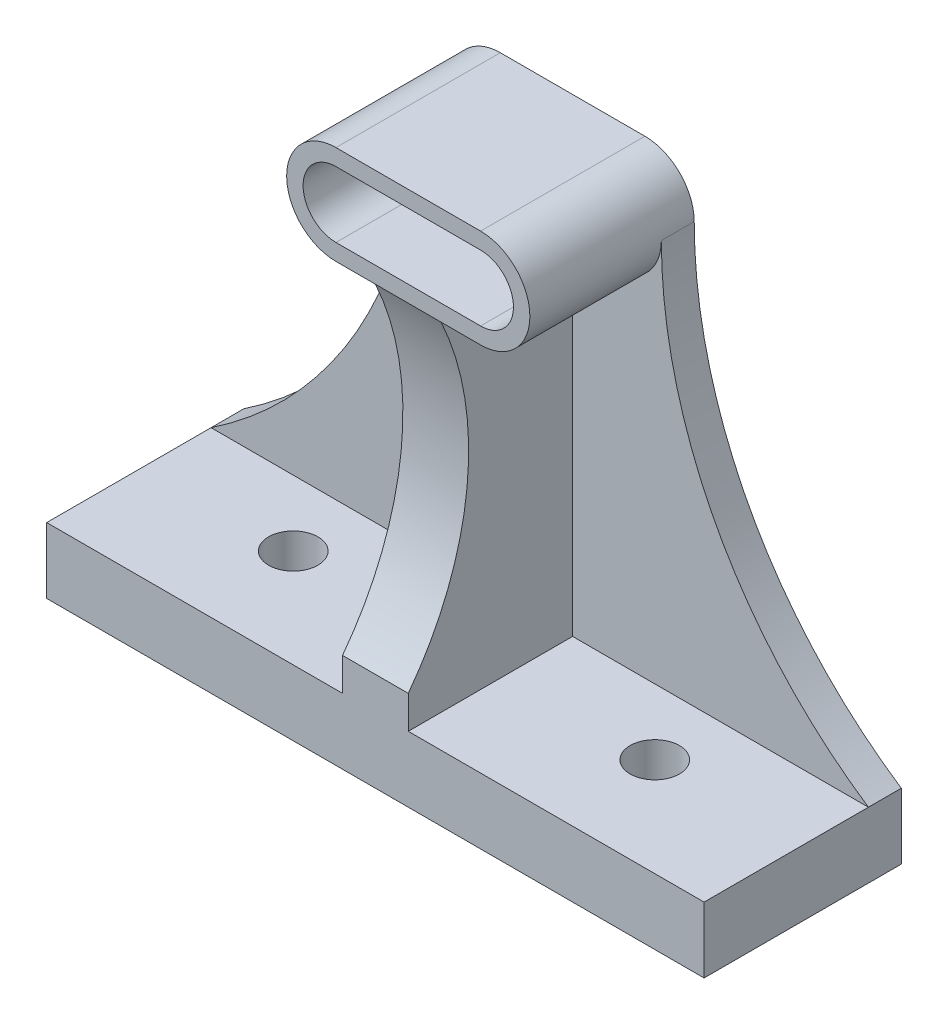
ISO-10303-21;
HEADER;
FILE_DESCRIPTION(('STEP AP214'),'2;1');
FILE_NAME('part.step','',(''),(''),'','','');
FILE_SCHEMA(('AUTOMOTIVE_DESIGN { 1 0 10303 214 1 1 1 1 }'));
ENDSEC;
DATA;
#1=APPLICATION_CONTEXT('core data for automotive mechanical design processes');
#2=APPLICATION_PROTOCOL_DEFINITION('international standard','automotive_design',2000,#1);
#3=PRODUCT_CONTEXT('',#1,'mechanical');
#4=PRODUCT('Part','Part','',(#3));
#5=PRODUCT_RELATED_PRODUCT_CATEGORY('part','',(#4));
#6=PRODUCT_DEFINITION_FORMATION('','',#4);
#7=PRODUCT_DEFINITION_CONTEXT('part definition',#1,'design');
#8=PRODUCT_DEFINITION('design','',#6,#7);
#9=PRODUCT_DEFINITION_SHAPE('','',#8);
#10=(LENGTH_UNIT() NAMED_UNIT(*) SI_UNIT(.MILLI.,.METRE.));
#11=(NAMED_UNIT(*) PLANE_ANGLE_UNIT() SI_UNIT($,.RADIAN.));
#12=(NAMED_UNIT(*) SI_UNIT($,.STERADIAN.) SOLID_ANGLE_UNIT());
#13=UNCERTAINTY_MEASURE_WITH_UNIT(LENGTH_MEASURE(1.E-05),#10,'distance_accuracy_value','');
#14=(GEOMETRIC_REPRESENTATION_CONTEXT(3) GLOBAL_UNCERTAINTY_ASSIGNED_CONTEXT((#13)) GLOBAL_UNIT_ASSIGNED_CONTEXT((#10,
#11,#12)) REPRESENTATION_CONTEXT('',''));
#15=CARTESIAN_POINT('',(0.,0.,0.));
#16=DIRECTION('',(0.,0.,1.));
#17=DIRECTION('',(1.,0.,0.));
#18=AXIS2_PLACEMENT_3D('',#15,#16,#17);
#19=CARTESIAN_POINT('',(39.,68.9,5.));
#20=DIRECTION('',(0.,0.,1.));
#21=DIRECTION('',(1.,0.,0.));
#22=AXIS2_PLACEMENT_3D('',#19,#20,#21);
#23=PLANE('',#22);
#24=DIRECTION('',(0.,-1.,0.));
#25=VECTOR('',#24,1.);
#26=CARTESIAN_POINT('',(45.,15.,5.));
#27=LINE('',#26,#25);
#28=CARTESIAN_POINT('',(45.,61.4,5.));
#29=VERTEX_POINT('',#28);
#30=CARTESIAN_POINT('',(45.,10.,5.));
#31=VERTEX_POINT('',#30);
#32=EDGE_CURVE('E194',#29,#31,#27,.T.);
#33=ORIENTED_EDGE('',*,*,#32,.F.);
#34=DIRECTION('',(-1.,0.,0.));
#35=VECTOR('',#34,1.);
#36=CARTESIAN_POINT('',(39.,61.4,5.));
#37=LINE('',#36,#35);
#38=CARTESIAN_POINT('',(39.,61.4,5.));
#39=VERTEX_POINT('',#38);
#40=EDGE_CURVE('E305',#29,#39,#37,.T.);
#41=ORIENTED_EDGE('',*,*,#40,.T.);
#42=CARTESIAN_POINT('',(39.,68.9,5.));
#43=DIRECTION('',(0.,0.,-1.));
#44=DIRECTION('',(1.,0.,0.));
#45=AXIS2_PLACEMENT_3D('',#42,#43,#44);
#46=CIRCLE('',#45,7.49999999999999);
#47=CARTESIAN_POINT('',(31.5,68.9,5.));
#48=VERTEX_POINT('',#47);
#49=EDGE_CURVE('E281',#39,#48,#46,.T.);
#50=ORIENTED_EDGE('',*,*,#49,.T.);
#51=CARTESIAN_POINT('',(-39.3168253968254,68.9,5.));
#52=DIRECTION('',(0.,0.,-1.));
#53=DIRECTION('',(-1.,0.,0.));
#54=AXIS2_PLACEMENT_3D('',#51,#52,#53);
#55=CIRCLE('',#54,70.8168253968254);
#56=CARTESIAN_POINT('',(0.,10.,5.));
#57=VERTEX_POINT('',#56);
#58=EDGE_CURVE('E288',#48,#57,#55,.T.);
#59=ORIENTED_EDGE('',*,*,#58,.T.);
#60=DIRECTION('',(1.,0.,0.));
#61=VECTOR('',#60,1.);
#62=CARTESIAN_POINT('',(0.,10.,5.));
#63=LINE('',#62,#61);
#64=EDGE_CURVE('E291',#57,#31,#63,.T.);
#65=ORIENTED_EDGE('',*,*,#64,.T.);
#66=EDGE_LOOP('',(#33,#41,#50,#59,#65));
#67=FACE_BOUND('',#66,.T.);
#68=ADVANCED_FACE('F44',(#67),#23,.T.);
#69=CARTESIAN_POINT('',(39.,61.4,25.));
#70=DIRECTION('',(0.,1.,0.));
#71=DIRECTION('',(-1.,0.,0.));
#72=AXIS2_PLACEMENT_3D('',#69,#70,#71);
#73=PLANE('',#72);
#74=DIRECTION('',(0.,0.,-1.));
#75=VECTOR('',#74,1.);
#76=CARTESIAN_POINT('',(45.,61.4,25.));
#77=LINE('',#76,#75);
#78=CARTESIAN_POINT('',(45.,61.4,25.));
#79=VERTEX_POINT('',#78);
#80=EDGE_CURVE('E67',#79,#29,#77,.T.);
#81=ORIENTED_EDGE('',*,*,#80,.F.);
#82=DIRECTION('',(1.,0.,0.));
#83=VECTOR('',#82,1.);
#84=CARTESIAN_POINT('',(39.,61.4,25.));
#85=LINE('',#84,#83);
#86=CARTESIAN_POINT('',(39.,61.4,25.));
#87=VERTEX_POINT('',#86);
#88=EDGE_CURVE('E262',#87,#79,#85,.T.);
#89=ORIENTED_EDGE('',*,*,#88,.F.);
#90=DIRECTION('',(0.,0.,-1.));
#91=VECTOR('',#90,1.);
#92=CARTESIAN_POINT('',(39.,61.4,25.));
#93=LINE('',#92,#91);
#94=EDGE_CURVE('E283',#87,#39,#93,.T.);
#95=ORIENTED_EDGE('',*,*,#94,.T.);
#96=ORIENTED_EDGE('',*,*,#40,.F.);
#97=EDGE_LOOP('',(#81,#89,#95,#96));
#98=FACE_BOUND('',#97,.T.);
#99=ADVANCED_FACE('F398',(#98),#73,.F.);
#100=CARTESIAN_POINT('',(100.,10.,30.));
#101=DIRECTION('',(0.,-1.,0.));
#102=DIRECTION('',(0.,0.,-1.));
#103=AXIS2_PLACEMENT_3D('',#100,#101,#102);
#104=PLANE('',#103);
#105=CARTESIAN_POINT('',(77.5,10.,15.));
#106=DIRECTION('',(0.,-1.,0.));
#107=DIRECTION('',(0.,0.,1.));
#108=AXIS2_PLACEMENT_3D('',#105,#106,#107);
#109=CIRCLE('',#108,3.75);
#110=CARTESIAN_POINT('',(77.5,10.,18.75));
#111=VERTEX_POINT('',#110);
#112=EDGE_CURVE('E454',#111,#111,#109,.T.);
#113=ORIENTED_EDGE('',*,*,#112,.T.);
#114=EDGE_LOOP('',(#113));
#115=FACE_BOUND('',#114,.T.);
#116=DIRECTION('',(0.,0.,-1.));
#117=VECTOR('',#116,1.);
#118=CARTESIAN_POINT('',(55.,10.,5.));
#119=LINE('',#118,#117);
#120=CARTESIAN_POINT('',(55.,10.,30.));
#121=VERTEX_POINT('',#120);
#122=CARTESIAN_POINT('',(55.,10.,5.));
#123=VERTEX_POINT('',#122);
#124=EDGE_CURVE('E220',#121,#123,#119,.T.);
#125=ORIENTED_EDGE('',*,*,#124,.F.);
#126=DIRECTION('',(-1.,0.,0.));
#127=VECTOR('',#126,1.);
#128=CARTESIAN_POINT('',(100.,10.,30.));
#129=LINE('',#128,#127);
#130=CARTESIAN_POINT('',(100.,10.,30.));
#131=VERTEX_POINT('',#130);
#132=EDGE_CURVE('E326',#131,#121,#129,.T.);
#133=ORIENTED_EDGE('',*,*,#132,.F.);
#134=DIRECTION('',(0.,0.,-1.));
#135=VECTOR('',#134,1.);
#136=CARTESIAN_POINT('',(100.,10.,30.));
#137=LINE('',#136,#135);
#138=CARTESIAN_POINT('',(100.,10.,5.));
#139=VERTEX_POINT('',#138);
#140=EDGE_CURVE('E338',#131,#139,#137,.T.);
#141=ORIENTED_EDGE('',*,*,#140,.T.);
#142=EDGE_CURVE('E292',#123,#139,#63,.T.);
#143=ORIENTED_EDGE('',*,*,#142,.F.);
#144=EDGE_LOOP('',(#125,#133,#141,#143));
#145=FACE_BOUND('',#144,.T.);
#146=ADVANCED_FACE('F362',(#115,#145),#104,.F.);
#147=CARTESIAN_POINT('',(22.5,10.,15.));
#148=DIRECTION('',(0.,1.,0.));
#149=DIRECTION('',(0.,0.,1.));
#150=AXIS2_PLACEMENT_3D('',#147,#148,#149);
#151=CIRCLE('',#150,3.75);
#152=CARTESIAN_POINT('',(22.5,10.,18.75));
#153=VERTEX_POINT('',#152);
#154=EDGE_CURVE('E215',#153,#153,#151,.T.);
#155=ORIENTED_EDGE('',*,*,#154,.F.);
#156=EDGE_LOOP('',(#155));
#157=FACE_BOUND('',#156,.T.);
#158=DIRECTION('',(0.,0.,1.));
#159=VECTOR('',#158,1.);
#160=CARTESIAN_POINT('',(45.,10.,30.));
#161=LINE('',#160,#159);
#162=CARTESIAN_POINT('',(45.,10.,30.));
#163=VERTEX_POINT('',#162);
#164=EDGE_CURVE('E188',#31,#163,#161,.T.);
#165=ORIENTED_EDGE('',*,*,#164,.F.);
#166=ORIENTED_EDGE('',*,*,#64,.F.);
#167=DIRECTION('',(0.,0.,-1.));
#168=VECTOR('',#167,1.);
#169=CARTESIAN_POINT('',(0.,10.,30.));
#170=LINE('',#169,#168);
#171=CARTESIAN_POINT('',(0.,10.,30.));
#172=VERTEX_POINT('',#171);
#173=EDGE_CURVE('E335',#172,#57,#170,.T.);
#174=ORIENTED_EDGE('',*,*,#173,.F.);
#175=EDGE_CURVE('E330',#163,#172,#129,.T.);
#176=ORIENTED_EDGE('',*,*,#175,.F.);
#177=EDGE_LOOP('',(#165,#166,#174,#176));
#178=FACE_BOUND('',#177,.T.);
#179=ADVANCED_FACE('F418',(#157,#178),#104,.F.);
#180=CARTESIAN_POINT('',(61.,61.4,5.));
#181=VERTEX_POINT('',#180);
#182=CARTESIAN_POINT('',(55.,61.4,5.));
#183=VERTEX_POINT('',#182);
#184=EDGE_CURVE('E303',#181,#183,#37,.T.);
#185=ORIENTED_EDGE('',*,*,#184,.T.);
#186=DIRECTION('',(0.,-1.,0.));
#187=VECTOR('',#186,1.);
#188=CARTESIAN_POINT('',(55.,15.,5.));
#189=LINE('',#188,#187);
#190=EDGE_CURVE('E222',#183,#123,#189,.T.);
#191=ORIENTED_EDGE('',*,*,#190,.T.);
#192=ORIENTED_EDGE('',*,*,#142,.T.);
#193=CARTESIAN_POINT('',(139.316825396825,68.9,5.));
#194=DIRECTION('',(0.,0.,-1.));
#195=DIRECTION('',(1.,0.,0.));
#196=AXIS2_PLACEMENT_3D('',#193,#194,#195);
#197=CIRCLE('',#196,70.8168253968254);
#198=CARTESIAN_POINT('',(68.5,68.9,5.));
#199=VERTEX_POINT('',#198);
#200=EDGE_CURVE('E298',#139,#199,#197,.T.);
#201=ORIENTED_EDGE('',*,*,#200,.T.);
#202=CARTESIAN_POINT('',(61.,68.9,5.));
#203=DIRECTION('',(0.,0.,-1.));
#204=DIRECTION('',(1.,0.,0.));
#205=AXIS2_PLACEMENT_3D('',#202,#203,#204);
#206=CIRCLE('',#205,7.49999999999999);
#207=EDGE_CURVE('E299',#199,#181,#206,.T.);
#208=ORIENTED_EDGE('',*,*,#207,.T.);
#209=EDGE_LOOP('',(#185,#191,#192,#201,#208));
#210=FACE_BOUND('',#209,.T.);
#211=ADVANCED_FACE('F393',(#210),#23,.T.);
#212=CARTESIAN_POINT('',(0.,10.,30.));
#213=DIRECTION('',(1.,0.,0.));
#214=DIRECTION('',(0.,0.,-1.));
#215=AXIS2_PLACEMENT_3D('',#212,#213,#214);
#216=PLANE('',#215);
#217=DIRECTION('',(0.,-1.,0.));
#218=VECTOR('',#217,1.);
#219=CARTESIAN_POINT('',(0.,10.,0.));
#220=LINE('',#219,#218);
#221=CARTESIAN_POINT('',(0.,10.,0.));
#222=VERTEX_POINT('',#221);
#223=CARTESIAN_POINT('',(0.,0.,0.));
#224=VERTEX_POINT('',#223);
#225=EDGE_CURVE('E318',#222,#224,#220,.T.);
#226=ORIENTED_EDGE('',*,*,#225,.T.);
#227=DIRECTION('',(0.,0.,-1.));
#228=VECTOR('',#227,1.);
#229=CARTESIAN_POINT('',(0.,0.,30.));
#230=LINE('',#229,#228);
#231=CARTESIAN_POINT('',(0.,0.,30.));
#232=VERTEX_POINT('',#231);
#233=EDGE_CURVE('E11',#232,#224,#230,.T.);
#234=ORIENTED_EDGE('',*,*,#233,.F.);
#235=DIRECTION('',(0.,-1.,0.));
#236=VECTOR('',#235,1.);
#237=CARTESIAN_POINT('',(0.,10.,30.));
#238=LINE('',#237,#236);
#239=EDGE_CURVE('E322',#172,#232,#238,.T.);
#240=ORIENTED_EDGE('',*,*,#239,.F.);
#241=ORIENTED_EDGE('',*,*,#173,.T.);
#242=DIRECTION('',(0.,0.,-1.));
#243=VECTOR('',#242,1.);
#244=CARTESIAN_POINT('',(0.,9.99999999999999,5.));
#245=LINE('',#244,#243);
#246=EDGE_CURVE('E314',#57,#222,#245,.T.);
#247=ORIENTED_EDGE('',*,*,#246,.T.);
#248=EDGE_LOOP('',(#226,#234,#240,#241,#247));
#249=FACE_BOUND('',#248,.T.);
#250=ADVANCED_FACE('F50',(#249),#216,.F.);
#251=CARTESIAN_POINT('',(0.,0.,30.));
#252=DIRECTION('',(0.,1.,0.));
#253=DIRECTION('',(0.,0.,1.));
#254=AXIS2_PLACEMENT_3D('',#251,#252,#253);
#255=PLANE('',#254);
#256=CARTESIAN_POINT('',(77.5,0.,15.));
#257=DIRECTION('',(0.,-1.,0.));
#258=DIRECTION('',(0.,0.,1.));
#259=AXIS2_PLACEMENT_3D('',#256,#257,#258);
#260=CIRCLE('',#259,3.75);
#261=CARTESIAN_POINT('',(77.5,0.,18.75));
#262=VERTEX_POINT('',#261);
#263=EDGE_CURVE('E443',#262,#262,#260,.T.);
#264=ORIENTED_EDGE('',*,*,#263,.F.);
#265=EDGE_LOOP('',(#264));
#266=FACE_BOUND('',#265,.T.);
#267=CARTESIAN_POINT('',(22.5,0.,15.));
#268=DIRECTION('',(0.,1.,0.));
#269=DIRECTION('',(0.,0.,1.));
#270=AXIS2_PLACEMENT_3D('',#267,#268,#269);
#271=CIRCLE('',#270,3.75);
#272=CARTESIAN_POINT('',(22.5,0.,18.75));
#273=VERTEX_POINT('',#272);
#274=EDGE_CURVE('E206',#273,#273,#271,.T.);
#275=ORIENTED_EDGE('',*,*,#274,.T.);
#276=EDGE_LOOP('',(#275));
#277=FACE_BOUND('',#276,.T.);
#278=DIRECTION('',(0.,0.,-1.));
#279=VECTOR('',#278,1.);
#280=CARTESIAN_POINT('',(100.,0.,30.));
#281=LINE('',#280,#279);
#282=CARTESIAN_POINT('',(100.,0.,30.));
#283=VERTEX_POINT('',#282);
#284=CARTESIAN_POINT('',(100.,0.,0.));
#285=VERTEX_POINT('',#284);
#286=EDGE_CURVE('E52',#283,#285,#281,.T.);
#287=ORIENTED_EDGE('',*,*,#286,.F.);
#288=DIRECTION('',(1.,0.,0.));
#289=VECTOR('',#288,1.);
#290=CARTESIAN_POINT('',(0.,0.,30.));
#291=LINE('',#290,#289);
#292=EDGE_CURVE('E321',#232,#283,#291,.T.);
#293=ORIENTED_EDGE('',*,*,#292,.F.);
#294=ORIENTED_EDGE('',*,*,#233,.T.);
#295=DIRECTION('',(1.,0.,0.));
#296=VECTOR('',#295,1.);
#297=CARTESIAN_POINT('',(0.,0.,0.));
#298=LINE('',#297,#296);
#299=EDGE_CURVE('E334',#224,#285,#298,.T.);
#300=ORIENTED_EDGE('',*,*,#299,.T.);
#301=EDGE_LOOP('',(#287,#293,#294,#300));
#302=FACE_BOUND('',#301,.T.);
#303=ADVANCED_FACE('F368',(#266,#277,#302),#255,.F.);
#304=CARTESIAN_POINT('',(100.,0.,30.));
#305=DIRECTION('',(-1.,0.,0.));
#306=DIRECTION('',(0.,0.,1.));
#307=AXIS2_PLACEMENT_3D('',#304,#305,#306);
#308=PLANE('',#307);
#309=DIRECTION('',(0.,1.,0.));
#310=VECTOR('',#309,1.);
#311=CARTESIAN_POINT('',(100.,0.,0.));
#312=LINE('',#311,#310);
#313=CARTESIAN_POINT('',(100.,10.,0.));
#314=VERTEX_POINT('',#313);
#315=EDGE_CURVE('E323',#285,#314,#312,.T.);
#316=ORIENTED_EDGE('',*,*,#315,.T.);
#317=DIRECTION('',(0.,0.,-1.));
#318=VECTOR('',#317,1.);
#319=CARTESIAN_POINT('',(100.,10.,5.));
#320=LINE('',#319,#318);
#321=EDGE_CURVE('E315',#139,#314,#320,.T.);
#322=ORIENTED_EDGE('',*,*,#321,.F.);
#323=ORIENTED_EDGE('',*,*,#140,.F.);
#324=DIRECTION('',(0.,1.,0.));
#325=VECTOR('',#324,1.);
#326=CARTESIAN_POINT('',(100.,0.,30.));
#327=LINE('',#326,#325);
#328=EDGE_CURVE('E329',#283,#131,#327,.T.);
#329=ORIENTED_EDGE('',*,*,#328,.F.);
#330=ORIENTED_EDGE('',*,*,#286,.T.);
#331=EDGE_LOOP('',(#316,#322,#323,#329,#330));
#332=FACE_BOUND('',#331,.T.);
#333=ADVANCED_FACE('F349',(#332),#308,.F.);
#334=CARTESIAN_POINT('',(0.,0.,30.));
#335=DIRECTION('',(0.,0.,1.));
#336=DIRECTION('',(1.,0.,0.));
#337=AXIS2_PLACEMENT_3D('',#334,#335,#336);
#338=PLANE('',#337);
#339=ORIENTED_EDGE('',*,*,#132,.T.);
#340=DIRECTION('',(0.,-1.,0.));
#341=VECTOR('',#340,1.);
#342=CARTESIAN_POINT('',(55.,15.,30.));
#343=LINE('',#342,#341);
#344=CARTESIAN_POINT('',(55.,15.,30.));
#345=VERTEX_POINT('',#344);
#346=EDGE_CURVE('E200',#345,#121,#343,.T.);
#347=ORIENTED_EDGE('',*,*,#346,.F.);
#348=DIRECTION('',(1.,0.,0.));
#349=VECTOR('',#348,1.);
#350=CARTESIAN_POINT('',(55.,15.,30.));
#351=LINE('',#350,#349);
#352=CARTESIAN_POINT('',(45.,15.,30.));
#353=VERTEX_POINT('',#352);
#354=EDGE_CURVE('E191',#353,#345,#351,.T.);
#355=ORIENTED_EDGE('',*,*,#354,.F.);
#356=DIRECTION('',(0.,-1.,0.));
#357=VECTOR('',#356,1.);
#358=CARTESIAN_POINT('',(45.,15.,30.));
#359=LINE('',#358,#357);
#360=EDGE_CURVE('E183',#353,#163,#359,.T.);
#361=ORIENTED_EDGE('',*,*,#360,.T.);
#362=ORIENTED_EDGE('',*,*,#175,.T.);
#363=ORIENTED_EDGE('',*,*,#239,.T.);
#364=ORIENTED_EDGE('',*,*,#292,.T.);
#365=ORIENTED_EDGE('',*,*,#328,.T.);
#366=EDGE_LOOP('',(#339,#347,#355,#361,#362,#363,#364,#365));
#367=FACE_BOUND('',#366,.T.);
#368=ADVANCED_FACE('F197',(#367),#338,.T.);
#369=CARTESIAN_POINT('',(0.,0.,0.));
#370=DIRECTION('',(0.,0.,1.));
#371=DIRECTION('',(1.,0.,0.));
#372=AXIS2_PLACEMENT_3D('',#369,#370,#371);
#373=PLANE('',#372);
#374=DIRECTION('',(1.,0.,0.));
#375=VECTOR('',#374,1.);
#376=CARTESIAN_POINT('',(39.,63.9,0.));
#377=LINE('',#376,#375);
#378=CARTESIAN_POINT('',(39.,63.9,0.));
#379=VERTEX_POINT('',#378);
#380=CARTESIAN_POINT('',(61.,63.9,0.));
#381=VERTEX_POINT('',#380);
#382=EDGE_CURVE('E245',#379,#381,#377,.T.);
#383=ORIENTED_EDGE('',*,*,#382,.T.);
#384=CARTESIAN_POINT('',(61.,68.9,0.));
#385=DIRECTION('',(0.,0.,1.));
#386=DIRECTION('',(1.,0.,0.));
#387=AXIS2_PLACEMENT_3D('',#384,#385,#386);
#388=CIRCLE('',#387,5.);
#389=CARTESIAN_POINT('',(61.,73.9,0.));
#390=VERTEX_POINT('',#389);
#391=EDGE_CURVE('E242',#381,#390,#388,.T.);
#392=ORIENTED_EDGE('',*,*,#391,.T.);
#393=DIRECTION('',(-1.,0.,0.));
#394=VECTOR('',#393,1.);
#395=CARTESIAN_POINT('',(39.,73.9,0.));
#396=LINE('',#395,#394);
#397=CARTESIAN_POINT('',(39.,73.9,0.));
#398=VERTEX_POINT('',#397);
#399=EDGE_CURVE('E235',#390,#398,#396,.T.);
#400=ORIENTED_EDGE('',*,*,#399,.T.);
#401=CARTESIAN_POINT('',(39.,68.9,0.));
#402=DIRECTION('',(0.,0.,1.));
#403=DIRECTION('',(1.,0.,0.));
#404=AXIS2_PLACEMENT_3D('',#401,#402,#403);
#405=CIRCLE('',#404,5.);
#406=EDGE_CURVE('E226',#398,#379,#405,.T.);
#407=ORIENTED_EDGE('',*,*,#406,.T.);
#408=EDGE_LOOP('',(#383,#392,#400,#407));
#409=FACE_BOUND('',#408,.T.);
#410=ORIENTED_EDGE('',*,*,#315,.F.);
#411=ORIENTED_EDGE('',*,*,#299,.F.);
#412=ORIENTED_EDGE('',*,*,#225,.F.);
#413=CARTESIAN_POINT('',(-39.3168253968254,68.9,0.));
#414=DIRECTION('',(0.,0.,-1.));
#415=DIRECTION('',(-1.,0.,0.));
#416=AXIS2_PLACEMENT_3D('',#413,#414,#415);
#417=CIRCLE('',#416,70.8168253968254);
#418=CARTESIAN_POINT('',(31.5,68.9,0.));
#419=VERTEX_POINT('',#418);
#420=EDGE_CURVE('E285',#419,#222,#417,.T.);
#421=ORIENTED_EDGE('',*,*,#420,.F.);
#422=CARTESIAN_POINT('',(39.,68.9,0.));
#423=DIRECTION('',(0.,0.,1.));
#424=DIRECTION('',(1.,0.,0.));
#425=AXIS2_PLACEMENT_3D('',#422,#423,#424);
#426=CIRCLE('',#425,7.49999999999999);
#427=CARTESIAN_POINT('',(39.,76.4,0.));
#428=VERTEX_POINT('',#427);
#429=EDGE_CURVE('E259',#428,#419,#426,.T.);
#430=ORIENTED_EDGE('',*,*,#429,.F.);
#431=DIRECTION('',(-1.,0.,0.));
#432=VECTOR('',#431,1.);
#433=CARTESIAN_POINT('',(39.,76.4,0.));
#434=LINE('',#433,#432);
#435=CARTESIAN_POINT('',(61.,76.4,0.));
#436=VERTEX_POINT('',#435);
#437=EDGE_CURVE('E264',#436,#428,#434,.T.);
#438=ORIENTED_EDGE('',*,*,#437,.F.);
#439=CARTESIAN_POINT('',(61.,68.9,0.));
#440=DIRECTION('',(0.,0.,1.));
#441=DIRECTION('',(1.,0.,0.));
#442=AXIS2_PLACEMENT_3D('',#439,#440,#441);
#443=CIRCLE('',#442,7.49999999999999);
#444=CARTESIAN_POINT('',(68.5,68.9,0.));
#445=VERTEX_POINT('',#444);
#446=EDGE_CURVE('E272',#445,#436,#443,.T.);
#447=ORIENTED_EDGE('',*,*,#446,.F.);
#448=CARTESIAN_POINT('',(139.316825396825,68.9,0.));
#449=DIRECTION('',(0.,0.,-1.));
#450=DIRECTION('',(1.,0.,0.));
#451=AXIS2_PLACEMENT_3D('',#448,#449,#450);
#452=CIRCLE('',#451,70.8168253968254);
#453=EDGE_CURVE('E287',#314,#445,#452,.T.);
#454=ORIENTED_EDGE('',*,*,#453,.F.);
#455=EDGE_LOOP('',(#410,#411,#412,#421,#430,#438,#447,#454));
#456=FACE_BOUND('',#455,.T.);
#457=ADVANCED_FACE('F353',(#409,#456),#373,.F.);
#458=CARTESIAN_POINT('',(-39.3168253968254,68.9,5.));
#459=DIRECTION('',(0.,0.,-1.));
#460=DIRECTION('',(-1.,0.,0.));
#461=AXIS2_PLACEMENT_3D('',#458,#459,#460);
#462=CYLINDRICAL_SURFACE('',#461,70.8168253968254);
#463=ORIENTED_EDGE('',*,*,#420,.T.);
#464=ORIENTED_EDGE('',*,*,#246,.F.);
#465=ORIENTED_EDGE('',*,*,#58,.F.);
#466=DIRECTION('',(0.,0.,-1.));
#467=VECTOR('',#466,1.);
#468=CARTESIAN_POINT('',(31.5,68.9,5.));
#469=LINE('',#468,#467);
#470=EDGE_CURVE('E320',#48,#419,#469,.T.);
#471=ORIENTED_EDGE('',*,*,#470,.T.);
#472=EDGE_LOOP('',(#463,#464,#465,#471));
#473=FACE_BOUND('',#472,.T.);
#474=ADVANCED_FACE('F372',(#473),#462,.F.);
#475=CARTESIAN_POINT('',(139.316825396825,68.9,5.));
#476=DIRECTION('',(0.,0.,-1.));
#477=DIRECTION('',(-1.,0.,0.));
#478=AXIS2_PLACEMENT_3D('',#475,#476,#477);
#479=CYLINDRICAL_SURFACE('',#478,70.8168253968254);
#480=ORIENTED_EDGE('',*,*,#453,.T.);
#481=DIRECTION('',(0.,0.,-1.));
#482=VECTOR('',#481,1.);
#483=CARTESIAN_POINT('',(68.5,68.9,5.));
#484=LINE('',#483,#482);
#485=EDGE_CURVE('E306',#199,#445,#484,.T.);
#486=ORIENTED_EDGE('',*,*,#485,.F.);
#487=ORIENTED_EDGE('',*,*,#200,.F.);
#488=ORIENTED_EDGE('',*,*,#321,.T.);
#489=EDGE_LOOP('',(#480,#486,#487,#488));
#490=FACE_BOUND('',#489,.T.);
#491=ADVANCED_FACE('F360',(#490),#479,.F.);
#492=CARTESIAN_POINT('',(61.,68.9,25.));
#493=DIRECTION('',(0.,0.,-1.));
#494=DIRECTION('',(-1.,0.,0.));
#495=AXIS2_PLACEMENT_3D('',#492,#493,#494);
#496=CYLINDRICAL_SURFACE('',#495,7.49999999999999);
#497=ORIENTED_EDGE('',*,*,#207,.F.);
#498=ORIENTED_EDGE('',*,*,#485,.T.);
#499=ORIENTED_EDGE('',*,*,#446,.T.);
#500=DIRECTION('',(0.,0.,-1.));
#501=VECTOR('',#500,1.);
#502=CARTESIAN_POINT('',(61.,76.4,25.));
#503=LINE('',#502,#501);
#504=CARTESIAN_POINT('',(61.,76.4,25.));
#505=VERTEX_POINT('',#504);
#506=EDGE_CURVE('E277',#505,#436,#503,.T.);
#507=ORIENTED_EDGE('',*,*,#506,.F.);
#508=CARTESIAN_POINT('',(61.,68.9,25.));
#509=DIRECTION('',(0.,0.,1.));
#510=DIRECTION('',(1.,0.,0.));
#511=AXIS2_PLACEMENT_3D('',#508,#509,#510);
#512=CIRCLE('',#511,7.49999999999999);
#513=CARTESIAN_POINT('',(61.,61.4,25.));
#514=VERTEX_POINT('',#513);
#515=EDGE_CURVE('E261',#514,#505,#512,.T.);
#516=ORIENTED_EDGE('',*,*,#515,.F.);
#517=DIRECTION('',(0.,0.,-1.));
#518=VECTOR('',#517,1.);
#519=CARTESIAN_POINT('',(61.,61.4,25.));
#520=LINE('',#519,#518);
#521=EDGE_CURVE('E276',#514,#181,#520,.T.);
#522=ORIENTED_EDGE('',*,*,#521,.T.);
#523=EDGE_LOOP('',(#497,#498,#499,#507,#516,#522));
#524=FACE_BOUND('',#523,.T.);
#525=ADVANCED_FACE('F389',(#524),#496,.T.);
#526=CARTESIAN_POINT('',(39.,68.9,25.));
#527=DIRECTION('',(0.,0.,1.));
#528=DIRECTION('',(1.,0.,0.));
#529=AXIS2_PLACEMENT_3D('',#526,#527,#528);
#530=PLANE('',#529);
#531=CARTESIAN_POINT('',(61.,68.9,25.));
#532=DIRECTION('',(0.,0.,1.));
#533=DIRECTION('',(1.,0.,0.));
#534=AXIS2_PLACEMENT_3D('',#531,#532,#533);
#535=CIRCLE('',#534,5.);
#536=CARTESIAN_POINT('',(61.,63.9,25.));
#537=VERTEX_POINT('',#536);
#538=CARTESIAN_POINT('',(61.,73.9,25.));
#539=VERTEX_POINT('',#538);
#540=EDGE_CURVE('E234',#537,#539,#535,.T.);
#541=ORIENTED_EDGE('',*,*,#540,.F.);
#542=DIRECTION('',(1.,0.,0.));
#543=VECTOR('',#542,1.);
#544=CARTESIAN_POINT('',(39.,63.9,25.));
#545=LINE('',#544,#543);
#546=CARTESIAN_POINT('',(39.,63.9,25.));
#547=VERTEX_POINT('',#546);
#548=EDGE_CURVE('E233',#547,#537,#545,.T.);
#549=ORIENTED_EDGE('',*,*,#548,.F.);
#550=CARTESIAN_POINT('',(39.,68.9,25.));
#551=DIRECTION('',(0.,0.,1.));
#552=DIRECTION('',(1.,0.,0.));
#553=AXIS2_PLACEMENT_3D('',#550,#551,#552);
#554=CIRCLE('',#553,5.);
#555=CARTESIAN_POINT('',(39.,73.9,25.));
#556=VERTEX_POINT('',#555);
#557=EDGE_CURVE('E230',#556,#547,#554,.T.);
#558=ORIENTED_EDGE('',*,*,#557,.F.);
#559=DIRECTION('',(-1.,0.,0.));
#560=VECTOR('',#559,1.);
#561=CARTESIAN_POINT('',(39.,73.9,25.));
#562=LINE('',#561,#560);
#563=EDGE_CURVE('E240',#539,#556,#562,.T.);
#564=ORIENTED_EDGE('',*,*,#563,.F.);
#565=EDGE_LOOP('',(#541,#549,#558,#564));
#566=FACE_BOUND('',#565,.T.);
#567=DIRECTION('',(1.,0.,0.));
#568=VECTOR('',#567,1.);
#569=CARTESIAN_POINT('',(50.,61.4,25.));
#570=LINE('',#569,#568);
#571=CARTESIAN_POINT('',(55.,61.4,25.));
#572=VERTEX_POINT('',#571);
#573=EDGE_CURVE('E207',#79,#572,#570,.T.);
#574=ORIENTED_EDGE('',*,*,#573,.T.);
#575=EDGE_CURVE('E58',#572,#514,#85,.T.);
#576=ORIENTED_EDGE('',*,*,#575,.T.);
#577=ORIENTED_EDGE('',*,*,#515,.T.);
#578=DIRECTION('',(-1.,0.,0.));
#579=VECTOR('',#578,1.);
#580=CARTESIAN_POINT('',(39.,76.4,25.));
#581=LINE('',#580,#579);
#582=CARTESIAN_POINT('',(39.,76.4,25.));
#583=VERTEX_POINT('',#582);
#584=EDGE_CURVE('E270',#505,#583,#581,.T.);
#585=ORIENTED_EDGE('',*,*,#584,.T.);
#586=CARTESIAN_POINT('',(39.,68.9,25.));
#587=DIRECTION('',(0.,0.,1.));
#588=DIRECTION('',(1.,0.,0.));
#589=AXIS2_PLACEMENT_3D('',#586,#587,#588);
#590=CIRCLE('',#589,7.49999999999999);
#591=EDGE_CURVE('E256',#583,#87,#590,.T.);
#592=ORIENTED_EDGE('',*,*,#591,.T.);
#593=ORIENTED_EDGE('',*,*,#88,.T.);
#594=EDGE_LOOP('',(#574,#576,#577,#585,#592,#593));
#595=FACE_BOUND('',#594,.T.);
#596=ADVANCED_FACE('F407',(#566,#595),#530,.T.);
#597=CARTESIAN_POINT('',(39.,68.9,25.));
#598=DIRECTION('',(0.,0.,-1.));
#599=DIRECTION('',(-1.,0.,0.));
#600=AXIS2_PLACEMENT_3D('',#597,#598,#599);
#601=CYLINDRICAL_SURFACE('',#600,7.49999999999999);
#602=ORIENTED_EDGE('',*,*,#470,.F.);
#603=ORIENTED_EDGE('',*,*,#49,.F.);
#604=ORIENTED_EDGE('',*,*,#94,.F.);
#605=ORIENTED_EDGE('',*,*,#591,.F.);
#606=DIRECTION('',(0.,0.,-1.));
#607=VECTOR('',#606,1.);
#608=CARTESIAN_POINT('',(39.,76.4,25.));
#609=LINE('',#608,#607);
#610=EDGE_CURVE('E267',#583,#428,#609,.T.);
#611=ORIENTED_EDGE('',*,*,#610,.T.);
#612=ORIENTED_EDGE('',*,*,#429,.T.);
#613=EDGE_LOOP('',(#602,#603,#604,#605,#611,#612));
#614=FACE_BOUND('',#613,.T.);
#615=ADVANCED_FACE('F377',(#614),#601,.T.);
#616=ORIENTED_EDGE('',*,*,#575,.F.);
#617=DIRECTION('',(0.,0.,-1.));
#618=VECTOR('',#617,1.);
#619=CARTESIAN_POINT('',(55.,61.4,25.));
#620=LINE('',#619,#618);
#621=EDGE_CURVE('E217',#572,#183,#620,.T.);
#622=ORIENTED_EDGE('',*,*,#621,.T.);
#623=ORIENTED_EDGE('',*,*,#184,.F.);
#624=ORIENTED_EDGE('',*,*,#521,.F.);
#625=EDGE_LOOP('',(#616,#622,#623,#624));
#626=FACE_BOUND('',#625,.T.);
#627=ADVANCED_FACE('F391',(#626),#73,.F.);
#628=CARTESIAN_POINT('',(39.,76.4,25.));
#629=DIRECTION('',(0.,-1.,0.));
#630=DIRECTION('',(0.,0.,-1.));
#631=AXIS2_PLACEMENT_3D('',#628,#629,#630);
#632=PLANE('',#631);
#633=ORIENTED_EDGE('',*,*,#437,.T.);
#634=ORIENTED_EDGE('',*,*,#610,.F.);
#635=ORIENTED_EDGE('',*,*,#584,.F.);
#636=ORIENTED_EDGE('',*,*,#506,.T.);
#637=EDGE_LOOP('',(#633,#634,#635,#636));
#638=FACE_BOUND('',#637,.T.);
#639=ADVANCED_FACE('F384',(#638),#632,.F.);
#640=CARTESIAN_POINT('',(39.,68.9,25.));
#641=DIRECTION('',(0.,0.,-1.));
#642=DIRECTION('',(-1.,0.,0.));
#643=AXIS2_PLACEMENT_3D('',#640,#641,#642);
#644=CYLINDRICAL_SURFACE('',#643,5.);
#645=ORIENTED_EDGE('',*,*,#406,.F.);
#646=DIRECTION('',(0.,0.,-1.));
#647=VECTOR('',#646,1.);
#648=CARTESIAN_POINT('',(39.,73.9,25.));
#649=LINE('',#648,#647);
#650=EDGE_CURVE('E237',#556,#398,#649,.T.);
#651=ORIENTED_EDGE('',*,*,#650,.F.);
#652=ORIENTED_EDGE('',*,*,#557,.T.);
#653=DIRECTION('',(0.,0.,-1.));
#654=VECTOR('',#653,1.);
#655=CARTESIAN_POINT('',(39.,63.9,25.));
#656=LINE('',#655,#654);
#657=EDGE_CURVE('E253',#547,#379,#656,.T.);
#658=ORIENTED_EDGE('',*,*,#657,.T.);
#659=EDGE_LOOP('',(#645,#651,#652,#658));
#660=FACE_BOUND('',#659,.T.);
#661=ADVANCED_FACE('F401',(#660),#644,.F.);
#662=CARTESIAN_POINT('',(39.,63.9,25.));
#663=DIRECTION('',(0.,1.,0.));
#664=DIRECTION('',(0.,0.,1.));
#665=AXIS2_PLACEMENT_3D('',#662,#663,#664);
#666=PLANE('',#665);
#667=DIRECTION('',(0.,0.,-1.));
#668=VECTOR('',#667,1.);
#669=CARTESIAN_POINT('',(61.,63.9,25.));
#670=LINE('',#669,#668);
#671=EDGE_CURVE('E255',#537,#381,#670,.T.);
#672=ORIENTED_EDGE('',*,*,#671,.T.);
#673=ORIENTED_EDGE('',*,*,#382,.F.);
#674=ORIENTED_EDGE('',*,*,#657,.F.);
#675=ORIENTED_EDGE('',*,*,#548,.T.);
#676=EDGE_LOOP('',(#672,#673,#674,#675));
#677=FACE_BOUND('',#676,.T.);
#678=ADVANCED_FACE('F477',(#677),#666,.T.);
#679=CARTESIAN_POINT('',(61.,68.9,25.));
#680=DIRECTION('',(0.,0.,-1.));
#681=DIRECTION('',(-1.,0.,0.));
#682=AXIS2_PLACEMENT_3D('',#679,#680,#681);
#683=CYLINDRICAL_SURFACE('',#682,5.);
#684=ORIENTED_EDGE('',*,*,#391,.F.);
#685=ORIENTED_EDGE('',*,*,#671,.F.);
#686=ORIENTED_EDGE('',*,*,#540,.T.);
#687=DIRECTION('',(0.,0.,-1.));
#688=VECTOR('',#687,1.);
#689=CARTESIAN_POINT('',(61.,73.9,25.));
#690=LINE('',#689,#688);
#691=EDGE_CURVE('E249',#539,#390,#690,.T.);
#692=ORIENTED_EDGE('',*,*,#691,.T.);
#693=EDGE_LOOP('',(#684,#685,#686,#692));
#694=FACE_BOUND('',#693,.T.);
#695=ADVANCED_FACE('F471',(#694),#683,.F.);
#696=CARTESIAN_POINT('',(39.,73.9,25.));
#697=DIRECTION('',(0.,-1.,0.));
#698=DIRECTION('',(0.,0.,-1.));
#699=AXIS2_PLACEMENT_3D('',#696,#697,#698);
#700=PLANE('',#699);
#701=ORIENTED_EDGE('',*,*,#563,.T.);
#702=ORIENTED_EDGE('',*,*,#650,.T.);
#703=ORIENTED_EDGE('',*,*,#399,.F.);
#704=ORIENTED_EDGE('',*,*,#691,.F.);
#705=EDGE_LOOP('',(#701,#702,#703,#704));
#706=FACE_BOUND('',#705,.T.);
#707=ADVANCED_FACE('F472',(#706),#700,.T.);
#708=CARTESIAN_POINT('',(55.,15.,5.));
#709=DIRECTION('',(-1.,0.,0.));
#710=DIRECTION('',(0.,0.,1.));
#711=AXIS2_PLACEMENT_3D('',#708,#709,#710);
#712=PLANE('',#711);
#713=ORIENTED_EDGE('',*,*,#124,.T.);
#714=ORIENTED_EDGE('',*,*,#190,.F.);
#715=ORIENTED_EDGE('',*,*,#621,.F.);
#716=CARTESIAN_POINT('',(55.,42.3686974456929,66.1855122960298));
#717=DIRECTION('',(-1.,0.,0.));
#718=DIRECTION('',(0.,0.,1.));
#719=AXIS2_PLACEMENT_3D('',#716,#717,#718);
#720=CIRCLE('',#719,45.37);
#721=EDGE_CURVE('E210',#572,#345,#720,.T.);
#722=ORIENTED_EDGE('',*,*,#721,.T.);
#723=ORIENTED_EDGE('',*,*,#346,.T.);
#724=EDGE_LOOP('',(#713,#714,#715,#722,#723));
#725=FACE_BOUND('',#724,.T.);
#726=ADVANCED_FACE('F395',(#725),#712,.F.);
#727=CARTESIAN_POINT('',(45.,15.,30.));
#728=DIRECTION('',(1.,0.,0.));
#729=DIRECTION('',(0.,0.,-1.));
#730=AXIS2_PLACEMENT_3D('',#727,#728,#729);
#731=PLANE('',#730);
#732=ORIENTED_EDGE('',*,*,#164,.T.);
#733=ORIENTED_EDGE('',*,*,#360,.F.);
#734=CARTESIAN_POINT('',(45.,42.3686974456929,66.1855122960298));
#735=DIRECTION('',(-1.,0.,0.));
#736=DIRECTION('',(0.,0.,1.));
#737=AXIS2_PLACEMENT_3D('',#734,#735,#736);
#738=CIRCLE('',#737,45.37);
#739=EDGE_CURVE('E189',#79,#353,#738,.T.);
#740=ORIENTED_EDGE('',*,*,#739,.F.);
#741=ORIENTED_EDGE('',*,*,#80,.T.);
#742=ORIENTED_EDGE('',*,*,#32,.T.);
#743=EDGE_LOOP('',(#732,#733,#740,#741,#742));
#744=FACE_BOUND('',#743,.T.);
#745=ADVANCED_FACE('F187',(#744),#731,.F.);
#746=CARTESIAN_POINT('',(50.,42.3686974456929,66.1855122960298));
#747=DIRECTION('',(-1.,0.,0.));
#748=DIRECTION('',(0.,0.,1.));
#749=AXIS2_PLACEMENT_3D('',#746,#747,#748);
#750=CYLINDRICAL_SURFACE('',#749,45.37);
#751=ORIENTED_EDGE('',*,*,#739,.T.);
#752=ORIENTED_EDGE('',*,*,#354,.T.);
#753=ORIENTED_EDGE('',*,*,#721,.F.);
#754=ORIENTED_EDGE('',*,*,#573,.F.);
#755=EDGE_LOOP('',(#751,#752,#753,#754));
#756=FACE_BOUND('',#755,.T.);
#757=ADVANCED_FACE('F204',(#756),#750,.F.);
#758=CARTESIAN_POINT('',(22.5,0.,15.));
#759=DIRECTION('',(0.,1.,0.));
#760=DIRECTION('',(0.,0.,1.));
#761=AXIS2_PLACEMENT_3D('',#758,#759,#760);
#762=CYLINDRICAL_SURFACE('',#761,3.75);
#763=ORIENTED_EDGE('',*,*,#274,.F.);
#764=EDGE_LOOP('',(#763));
#765=FACE_BOUND('',#764,.T.);
#766=ORIENTED_EDGE('',*,*,#154,.T.);
#767=EDGE_LOOP('',(#766));
#768=FACE_BOUND('',#767,.T.);
#769=ADVANCED_FACE('F450',(#765,#768),#762,.F.);
#770=CARTESIAN_POINT('',(77.5,0.,15.));
#771=DIRECTION('',(0.,1.,0.));
#772=DIRECTION('',(0.,0.,1.));
#773=AXIS2_PLACEMENT_3D('',#770,#771,#772);
#774=CYLINDRICAL_SURFACE('',#773,3.75);
#775=ORIENTED_EDGE('',*,*,#263,.T.);
#776=EDGE_LOOP('',(#775));
#777=FACE_BOUND('',#776,.T.);
#778=ORIENTED_EDGE('',*,*,#112,.F.);
#779=EDGE_LOOP('',(#778));
#780=FACE_BOUND('',#779,.T.);
#781=ADVANCED_FACE('F448',(#777,#780),#774,.F.);
#782=CLOSED_SHELL('',(#68,#99,#146,#179,#211,#250,#303,#333,#368,#457,#474,#491,#525,#596,#615,
#627,#639,#661,#678,#695,#707,#726,#745,#757,#769,#781));
#783=MANIFOLD_SOLID_BREP('B2',#782);
#784=ADVANCED_BREP_SHAPE_REPRESENTATION('',(#18,#783),#14);
#785=SHAPE_DEFINITION_REPRESENTATION(#9,#784);
ENDSEC;
END-ISO-10303-21;
